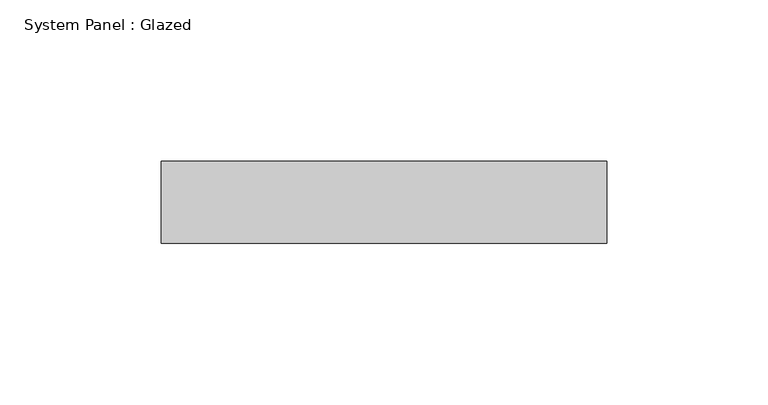
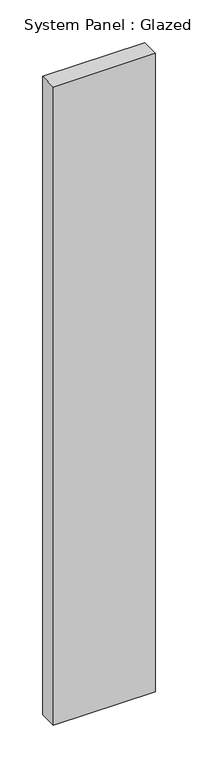
"""IFC4 building model written with IfcOpenShell, lengths in millimetres: plate geometry, System Panel : Glazed."""

from ifc_helpers import new_model, si_unit, origin, origin_with_axes, place, context, project, spatial, polyline, outline, extrude, source, transform, mapped, element, save


def system_panel_glazed_22bcd51f(model_context):
    return source(origin(), model_context, "Body", "SweptSolid", [
        extrude(outline(polyline([(69.0796158, 19.05), (-69.0796158, 19.05), (-69.0796158, 44.45), (69.0796158, 44.45), (69.0796158, 19.05)])), origin_with_axes(), (0.0, 0.0, 1.0), 914.4),
    ])


if __name__ == "__main__":
    model = new_model("IFC4")
    model_context = context("Model", 3, world=origin())
    ifc_project = project(units=[si_unit("LENGTHUNIT", "METRE", prefix="MILLI")], contexts=[model_context])
    site = spatial("IfcSite", under=ifc_project)
    building = spatial("IfcBuilding", under=site)
    placement = place(None, origin())
    system_panel_glazed_shape = system_panel_glazed_22bcd51f(model_context)
    element("IfcPlate", 1, ObjectType="System Panel : Glazed", at=placement, inside=building, context=model_context, shape_type="MappedRepresentation", body=[
        mapped(system_panel_glazed_shape, transform((0.0, 0.0, 0.0), x_axis=(1.0, 0.0, 0.0), y_axis=(0.0, 1.0, 0.0), z_axis=(0.0, 0.0, 1.0))),
    ])
    save(model, "model.ifc")

# Revit data of these elements
# Type "System Panel : Glazed"
#   Construction Type Id = "GSP4R"
#   Analytic Construction = "1/8 in Pilkington single glazing"
#   Visual Light Transmittance = 0.9
#   Solar Heat Gain Coefficient = 0.86
#   Heat Transfer Coefficient (U) = 6.7069 W/(m²·K)
# Element 1 (IfcPlate, "System Panel : Glazed")
#   Materials on its faces: "Glass"
# Materials
#   "Glass": class "Glass", colour RGB 0 128 192, transparency 0.75, Description = "Soda Lime Glass", Cost = 0
